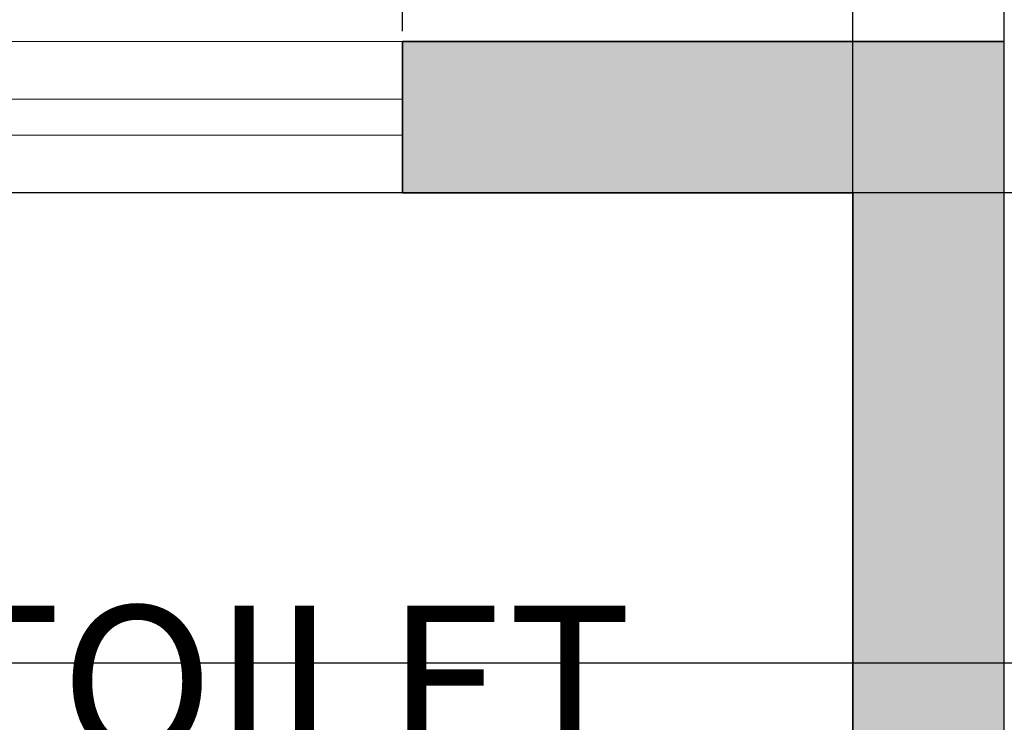
# Model space of a CAD drawing. Units: inches. Extents: x 2696 to 3240, y 1564 to 2310.
# Tile 62 of 76: x 2907 to 2966, y 2222 to 2264. Entities that reach past the tile are written whole.
import ezdxf

# ---------------------------------------------------------------- set-up
doc = ezdxf.new("R2010")
doc.units = ezdxf.units.IN
for name, color, linetype, lineweight in [('A-ANNO-DIMS', 3, 'Continuous', 18), ('A-AREA-IDEN', 7, 'Continuous', 18), ('A-WALL', 7, 'Continuous', 35), ('A-WALL-PATT', 9, 'Continuous', 13), ('WINDOW', 2, 'Continuous', 18)]:
    doc.layers.add(name, color=color, linetype=linetype, lineweight=lineweight)
doc.styles.add('TIMES NEW', font='times.ttf')
doc.styles.add('YQ_DIM', font='SUPEROS.SHX', dxfattribs={"width": 0.8, "bigfont": 'HZDX.SHX'})
doc.dimstyles.new('Siddhuu', dxfattribs={"dimtxt": 6, "dimasz": 2.5, "dimexe": 1.25, "dimexo": 0.625, "dimtad": 1, "dimdec": 1, "dimlunit": 4, "dimtxsty": 'TIMES NEW', "dimcen": 2.5, "dimclrd": 256, "dimclre": 1, "dimclrt": 7, "dimadec": 0, "dimazin": 0, "dimtfac": 1, "dimtdec": 1, "dimtmove": 0, "dimatfit": 3, "dimfxl": 1, "dimtolj": 1, "dimlwd": -1, "dimarcsym": 0})

# ---------------------------------------------------------------- blocks, each defined once
blk = doc.blocks.new('WD_WIN4')
for p, q in [((-0.5, 0.5), (0.5, 0.5)), ((-0.5, 0.12), (0.5, 0.12)), ((-0.5, -0.12), (0.5, -0.12)), ((-0.5, -0.5), (0.5, -0.5))]:
    blk.add_line(p, q)
blk = doc.blocks.new('*D9')
at = {"layer": 'A-ANNO-DIMS', "color": 0, "lineweight": -2, "transparency": 16777216}
for p, q in [((2745.611, 2262.826), (2745.611, 2282.188)), ((3199.611, 2262.826), (3199.611, 2282.188))]:
    blk.add_line(p, q, dxfattribs=at)
at = {"layer": 'A-ANNO-DIMS', "color": 0, "transparency": 16777216}
blk.add_line((2757.611, 2280.938), (3187.611, 2280.938), dxfattribs=at)
for points in [[(2757.611, 2282.938), (2757.611, 2278.938), (2745.611, 2280.938)], [(3187.611, 2282.938), (3187.611, 2278.938), (3199.611, 2280.938)]]:
    blk.add_solid(points, dxfattribs=at)
at = {"layer": 'Defpoints', "color": 0, "transparency": 16777216}
for p in [(3199.611, 2280.938), (2745.611, 2262.201), (3199.611, 2262.201)]:
    blk.add_point(p, dxfattribs=at)
at = {"layer": 'A-ANNO-DIMS', "color": 0, "transparency": 16777216, "insert": (2972.611, 2290.718), "char_height": 18, "attachment_point": 5, "style": 'TIMES NEW'}
blk.add_mtext("\\A1;36'", dxfattribs=at)
blk = doc.blocks.new('*D20')
at = {"layer": 'A-ANNO-DIMS', "color": 1, "lineweight": -2, "transparency": 16777216}
for p, q in [((2905.91, 2262.826), (2905.91, 2267.051)), ((2929.91, 2262.826), (2929.91, 2267.051))]:
    blk.add_line(p, q, dxfattribs=at)
at = {"layer": 'A-ANNO-DIMS', "transparency": 16777216}
for p, q in [((2905.91, 2265.801), (2844.76, 2265.801)), ((2927.41, 2265.801), (2908.41, 2265.801))]:
    blk.add_line(p, q, dxfattribs=at)
for points in [[(2908.41, 2266.218), (2908.41, 2265.384), (2905.91, 2265.801)], [(2927.41, 2266.218), (2927.41, 2265.384), (2929.91, 2265.801)]]:
    blk.add_solid(points, dxfattribs=at)
at = {"layer": 'Defpoints', "color": 0, "transparency": 16777216}
for p in [(2905.91, 2265.801), (2905.91, 2262.201), (2929.91, 2262.201)]:
    blk.add_point(p, dxfattribs=at)
at = {"layer": 'A-ANNO-DIMS', "color": 7, "transparency": 16777216, "insert": (2874.085, 2269.493), "char_height": 6, "attachment_point": 5, "style": 'TIMES NEW'}
blk.add_mtext('\\A1;WINDOW 2\'-0"', dxfattribs=at)
blk = doc.blocks.new('*D59')
at = {"layer": 'A-ANNO-DIMS', "color": 1, "lineweight": -2, "transparency": 16777216}
for p, q in [((2884.709, 1740.826), (2884.709, 2298.451)), ((2956.709, 1740.826), (2956.709, 2298.451))]:
    blk.add_line(p, q, dxfattribs=at)
at = {"layer": 'A-ANNO-DIMS', "transparency": 16777216}
blk.add_line((2887.209, 2297.201), (2954.209, 2297.201), dxfattribs=at)
for points in [[(2887.209, 2297.618), (2887.209, 2296.784), (2884.709, 2297.201)], [(2954.209, 2297.618), (2954.209, 2296.784), (2956.709, 2297.201)]]:
    blk.add_solid(points, dxfattribs=at)
at = {"layer": 'Defpoints', "color": 0, "transparency": 16777216}
for p in [(2956.709, 2297.201), (2884.709, 1740.201), (2956.709, 1740.201)]:
    blk.add_point(p, dxfattribs=at)
at = {"layer": 'A-ANNO-DIMS', "color": 7, "transparency": 16777216, "insert": (2920.709, 2300.878), "char_height": 6, "attachment_point": 5, "style": 'TIMES NEW'}
blk.add_mtext('\\A1;6\'-0"', dxfattribs=at)
blk = doc.blocks.new('*D61')
at = {"layer": 'A-ANNO-DIMS', "color": 1, "lineweight": -2, "transparency": 16777216}
for p, q in [((2965.709, 2141.326), (2965.709, 2298.451)), ((3044.302, 2141.326), (3044.302, 2298.451))]:
    blk.add_line(p, q, dxfattribs=at)
at = {"layer": 'A-ANNO-DIMS', "transparency": 16777216}
blk.add_line((2968.209, 2297.201), (3041.802, 2297.201), dxfattribs=at)
for points in [[(2968.209, 2297.618), (2968.209, 2296.784), (2965.709, 2297.201)], [(3041.802, 2297.618), (3041.802, 2296.784), (3044.302, 2297.201)]]:
    blk.add_solid(points, dxfattribs=at)
at = {"layer": 'Defpoints', "color": 0, "transparency": 16777216}
for p in [(3044.302, 2297.201), (2965.709, 2140.701), (3044.302, 2140.701)]:
    blk.add_point(p, dxfattribs=at)
at = {"layer": 'A-ANNO-DIMS', "color": 7, "transparency": 16777216, "insert": (3005.005, 2300.962), "char_height": 6, "attachment_point": 5, "style": 'TIMES NEW'}
blk.add_mtext('\\A1;6\'-6 1/2"', dxfattribs=at)
blk = doc.blocks.new('*D63')
at = {"layer": 'A-ANNO-DIMS', "color": 1, "lineweight": -2, "transparency": 16777216}
for p, q in [((2965.709, 1989.826), (2965.709, 2298.451)), ((3069.209, 1989.826), (3069.209, 2298.451))]:
    blk.add_line(p, q, dxfattribs=at)
at = {"layer": 'A-ANNO-DIMS', "transparency": 16777216}
blk.add_line((2968.209, 2297.201), (3066.709, 2297.201), dxfattribs=at)
for points in [[(2968.209, 2297.618), (2968.209, 2296.784), (2965.709, 2297.201)], [(3066.709, 2297.618), (3066.709, 2296.784), (3069.209, 2297.201)]]:
    blk.add_solid(points, dxfattribs=at)
at = {"layer": 'Defpoints', "color": 0, "transparency": 16777216}
for p in [(3069.209, 2297.201), (2965.709, 1989.201), (3069.209, 1989.201)]:
    blk.add_point(p, dxfattribs=at)
at = {"layer": 'A-ANNO-DIMS', "color": 7, "transparency": 16777216, "insert": (3017.459, 2300.962), "char_height": 6, "attachment_point": 5, "style": 'TIMES NEW'}
blk.add_mtext('\\A1;8\'-7 1/2"', dxfattribs=at)
blk = doc.blocks.new('*D70')
at = {"layer": 'A-ANNO-DIMS', "color": 1, "lineweight": -2, "transparency": 16777216}
for p, q in [((2929.91, 2262.826), (2929.91, 2298.451)), ((2965.709, 2262.826), (2965.709, 2298.451))]:
    blk.add_line(p, q, dxfattribs=at)
at = {"layer": 'A-ANNO-DIMS', "transparency": 16777216}
blk.add_line((2932.41, 2297.201), (2963.209, 2297.201), dxfattribs=at)
for points in [[(2932.41, 2297.618), (2932.41, 2296.784), (2929.91, 2297.201)], [(2963.209, 2297.618), (2963.209, 2296.784), (2965.709, 2297.201)]]:
    blk.add_solid(points, dxfattribs=at)
at = {"layer": 'Defpoints', "color": 0, "transparency": 16777216}
for p in [(2965.709, 2297.201), (2929.91, 2262.201), (2965.709, 2262.201)]:
    blk.add_point(p, dxfattribs=at)
at = {"layer": 'A-ANNO-DIMS', "color": 7, "transparency": 16777216, "insert": (2947.809, 2300.878), "char_height": 6, "attachment_point": 5, "style": 'TIMES NEW'}
blk.add_mtext('\\A1;3\'-0"', dxfattribs=at)
blk = doc.blocks.new('*D76')
at = {"layer": 'A-ANNO-DIMS', "color": 1, "lineweight": -2, "transparency": 16777216}
for p, q in [((3189.986, 2253.201), (2709.361, 2253.201)), ((3189.986, 2225.201), (2709.361, 2225.201))]:
    blk.add_line(p, q, dxfattribs=at)
at = {"layer": 'A-ANNO-DIMS', "transparency": 16777216}
blk.add_line((2710.611, 2250.701), (2710.611, 2227.701), dxfattribs=at)
for points in [[(2710.195, 2250.701), (2711.028, 2250.701), (2710.611, 2253.201)], [(2710.195, 2227.701), (2711.028, 2227.701), (2710.611, 2225.201)]]:
    blk.add_solid(points, dxfattribs=at)
at = {"layer": 'Defpoints', "color": 0, "transparency": 16777216}
for p in [(3190.611, 2253.201), (2710.611, 2225.201), (3190.611, 2225.201)]:
    blk.add_point(p, dxfattribs=at)
at = {"layer": 'A-ANNO-DIMS', "color": 7, "transparency": 16777216, "insert": (2706.986, 2239.201), "char_height": 6, "attachment_point": 5, "rotation": 90, "style": 'TIMES NEW'}
blk.add_mtext('\\A1;2\'-4"', dxfattribs=at)

msp = doc.modelspace()

# ---------------------------------------------------------------- hatches: boundary and pattern name
at = {"layer": 'A-WALL-PATT', "transparency": 33554556}
h = msp.add_hatch(color=256, dxfattribs=at)
h.dxf.hatch_style = 1
h.paths.add_polyline_path([(2879.111, 2253.201), (2905.91, 2253.201), (2905.91, 2262.201), (2841.889, 2262.201), (2841.889, 2253.201), (2870.111, 2253.201), (2870.111, 2176.601), (2965.709, 2176.601), (2965.709, 2206.701), (2973.583, 2206.701), (2973.583, 2215.701), (2965.709, 2215.701), (2965.709, 2262.201), (2929.91, 2262.201), (2929.91, 2253.201), (2956.709, 2253.201), (2956.709, 2185.601), (2879.111, 2185.601)])
h.paths.add_polyline_path([(2782.834, 2262.201), (2745.611, 2262.201), (2745.611, 2228.729), (2754.611, 2228.729), (2754.611, 2253.201), (2782.834, 2253.201)])
h.paths.add_polyline_path([(2754.611, 2136.201), (2965.709, 2136.201), (2965.709, 2145.201), (2879.111, 2145.201), (2879.111, 2147.074), (2877.34, 2147.074), (2870.111, 2147.074), (2870.111, 2145.201), (2754.611, 2145.201), (2754.611, 2169.674), (2745.611, 2169.674), (2745.611, 2000.201), (2754.611, 2000.201), (2754.611, 2019.201), (2849.083, 2019.201), (2849.083, 2023.701), (2841.209, 2023.701), (2841.209, 2051.827), (2836.709, 2051.827), (2836.709, 2023.701), (2754.611, 2023.701), (2754.611, 2091.201), (2836.709, 2091.201), (2836.709, 2087.827), (2841.209, 2087.827), (2841.209, 2095.701), (2754.611, 2095.701)])
h.paths.add_polyline_path([(2965.709, 2136.201), (2956.709, 2136.201), (2956.709, 2023.701), (2885.083, 2023.701), (2885.083, 2019.201), (2956.709, 2019.201), (2956.709, 1950.575), (2965.709, 1950.575), (2965.709, 1980.201), (2973.583, 1980.201), (2973.583, 1989.201), (2965.709, 1989.201)])
h.paths.add_polyline_path([(2754.611, 1906.701), (2880.209, 1906.701), (2884.709, 1906.701), (2956.709, 1906.701), (2956.709, 1792.701), (2944.709, 1792.701), (2944.709, 1783.701), (2956.709, 1783.701), (2956.709, 1740.201), (2884.709, 1740.201), (2884.709, 1783.701), (2896.709, 1783.701), (2896.709, 1792.701), (2884.709, 1792.701), (2884.709, 1846.701), (2880.209, 1846.701), (2880.209, 1740.201), (2754.611, 1740.201), (2754.611, 1777.201), (2745.611, 1777.201), (2745.611, 1692.701), (2754.611, 1692.701), (2754.611, 1731.201), (2956.709, 1731.201), (2956.709, 1723.327), (2965.709, 1723.327), (2965.709, 1884.201), (2973.583, 1884.201), (2973.583, 1893.201), (2965.709, 1893.201), (2965.709, 1914.575), (2956.709, 1914.575), (2956.709, 1911.201), (2754.611, 1911.201), (2754.611, 1930.201), (2745.611, 1930.201), (2745.611, 1817.201), (2754.611, 1817.201), (2754.611, 1854.201), (2826.611, 1854.201), (2826.611, 1868.827), (2822.111, 1868.827), (2822.111, 1858.701), (2754.611, 1858.701)])
h.paths.add_polyline_path([(2965.709, 1656.201), (3008.237, 1656.201), (3008.237, 1665.201), (2965.709, 1665.201), (2965.709, 1693.327), (2956.709, 1693.327), (2956.709, 1686.201), (2934.583, 1686.201), (2934.583, 1681.701), (2956.709, 1681.701), (2956.709, 1614.201), (2896.709, 1614.201), (2896.709, 1681.701), (2904.583, 1681.701), (2904.583, 1686.201), (2892.209, 1686.201), (2892.209, 1614.201), (2858.41, 1614.201), (2858.41, 1605.201), (2965.709, 1605.201)])
h.paths.add_polyline_path([(2788.41, 1614.201), (2754.611, 1614.201), (2754.611, 1652.701), (2745.611, 1652.701), (2745.611, 1605.201), (2788.41, 1605.201)])
h.paths.add_polyline_path([(3199.611, 1633.048), (3190.611, 1633.048), (3190.611, 1614.201), (3082.611, 1614.201), (3082.611, 1665.201), (3070.237, 1665.201), (3070.237, 1656.201), (3078.111, 1656.201), (3078.111, 1605.201), (3199.611, 1605.201)])
h.paths.add_polyline_path([(3199.611, 1702.048), (3190.611, 1702.048), (3190.611, 1699.701), (3106.611, 1699.701), (3106.611, 1747.701), (3190.611, 1747.701), (3190.611, 1752.201), (3082.611, 1752.201), (3082.611, 1760.075), (3078.111, 1760.075), (3078.111, 1747.701), (3102.111, 1747.701), (3102.111, 1699.701), (3078.111, 1699.701), (3078.111, 1695.201), (3190.611, 1695.201), (3190.611, 1676.355), (3199.611, 1676.355)])
h.paths.add_polyline_path([(3199.611, 1783.201), (3190.611, 1783.201), (3190.611, 1745.355), (3199.611, 1745.355)])
h.paths.add_polyline_path([(3082.611, 1884.201), (3190.611, 1884.201), (3190.611, 1853.201), (3199.611, 1853.201), (3199.611, 1901.701), (3190.611, 1901.701), (3190.611, 1893.201), (3005.583, 1893.201), (3005.583, 1891.281), (3005.583, 1884.201), (3078.111, 1884.201), (3078.111, 1792.075), (3082.611, 1792.075)])
h.paths.add_polyline_path([(3199.611, 1994.701), (3190.611, 1994.701), (3190.611, 1989.201), (3073.709, 1989.201), (3073.709, 2034.201), (3069.209, 2034.201), (3069.209, 1989.201), (3005.583, 1989.201), (3005.583, 1980.201), (3190.611, 1980.201), (3190.611, 1971.701), (3199.611, 1971.701)])
h.paths.add_polyline_path([(3199.611, 2155.201), (3190.611, 2155.201), (3190.611, 2064.701), (3199.611, 2064.701)])
h.paths.add_polyline_path([(3190.611, 2074.701), (3106.611, 2074.701), (3106.611, 2122.701), (3190.611, 2122.701), (3190.611, 2127.201), (3082.709, 2127.201), (3082.709, 2135.075), (3073.709, 2135.075), (3073.709, 2122.701), (3102.111, 2122.701), (3102.111, 2074.701), (3069.209, 2074.701), (3069.209, 2070.201), (3190.611, 2070.201)])
h.paths.add_polyline_path([(3082.709, 2253.201), (3190.611, 2253.201), (3190.611, 2225.201), (3199.611, 2225.201), (3199.611, 2262.201), (3073.709, 2262.201), (3073.709, 2215.701), (3035.583, 2215.701), (3035.583, 2206.701), (3073.709, 2206.701), (3073.709, 2171.075), (3082.709, 2171.075)])

# ---------------------------------------------------------------- linework, layer by layer
at = {"layer": 'A-WALL'}
for p, q in [((2929.91, 2262.201), (2929.91, 2253.201)), ((2929.91, 2262.201), (2965.709, 2262.201)), ((2929.91, 2253.201), (2929.91, 2262.201)), ((2929.91, 2253.201), (2956.709, 2253.201)), ((2956.709, 2185.601), (2956.709, 2253.201))]:
    msp.add_line(p, q, dxfattribs=at)

# ---------------------------------------------------------------- block references
at = {"layer": 'WINDOW', "xscale": 24, "yscale": 9, "zscale": 24, "rotation": 180}
msp.add_blockref('WD_WIN4', (2917.91, 2257.701), dxfattribs=at)

# ---------------------------------------------------------------- texts
at = {"layer": 'A-AREA-IDEN', "insert": (2902.228, 2228.623), "char_height": 9, "attachment_point": 1, "style": 'YQ_DIM'}
msp.add_mtext_dynamic_manual_height_columns('TOILET\\P5\'X5\'4.5"', width=48.00324, gutter_width=12.5, heights=[0], dxfattribs=at)

# ---------------------------------------------------------------- dimensions: what is measured, and where the dimension line sits
at = {"layer": 'A-ANNO-DIMS'}
for base, p1, p2, picture, middle in [((3044.302, 2297.201), (2965.709, 2140.701), (3044.302, 2140.701), '*D61', (3005.005, 2300.962)), ((3069.209, 2297.201), (2965.709, 1989.201), (3069.209, 1989.201), '*D63', (3017.459, 2300.962)), ((2956.709, 2297.201), (2884.709, 1740.201), (2956.709, 1740.201), '*D59', (2920.709, 2300.878)), ((2965.709, 2297.201), (2929.91, 2262.201), (2965.709, 2262.201), '*D70', (2947.809, 2300.878))]:
    dim = msp.add_linear_dim(base=base, p1=p1, p2=p2, dimstyle='Siddhuu', override={"dimdec": 1, "dimlfac": 1, "dimrnd": 0, "dimzin": 1, "dimdsep": 46, "dimlunit": 4, "dimfrac": 2}, dxfattribs=at)
    dim.commit()
    dim.dimension.update_dxf_attribs({"geometry": picture, "text_midpoint": middle})
dim = msp.add_linear_dim(base=(3199.611, 2280.938), p1=(2745.611, 2262.201), p2=(3199.611, 2262.201), text="36'", dimstyle='Siddhuu', override={"dimtxt": 18, "dimasz": 12, "dimclrd": 0, "dimclre": 0, "dimclrt": 0}, dxfattribs=at)
dim.commit()
dim.dimension.update_dxf_attribs({"geometry": '*D9', "text_midpoint": (2972.611, 2290.718)})
dim = msp.add_linear_dim(base=(2905.91, 2265.801), p1=(2929.91, 2262.201), p2=(2905.91, 2262.201), angle=180, text='WINDOW <>', dimstyle='Siddhuu', override={"dimdec": 1, "dimlfac": 1, "dimrnd": 0, "dimzin": 1, "dimdsep": 46, "dimlunit": 4, "dimfrac": 2}, dxfattribs=at)
dim.commit()
dim.dimension.update_dxf_attribs({"geometry": '*D20', "text_midpoint": (2874.085, 2269.493)})
dim = msp.add_linear_dim(base=(2710.611, 2225.201), p1=(3190.611, 2253.201), p2=(3190.611, 2225.201), angle=90, dimstyle='Siddhuu', override={"dimdec": 1, "dimlfac": 1, "dimrnd": 0, "dimzin": 1, "dimdsep": 46, "dimlunit": 4, "dimfrac": 2}, dxfattribs=at)
dim.commit()
dim.dimension.update_dxf_attribs({"geometry": '*D76', "text_midpoint": (2706.986, 2239.201)})

doc.saveas('drawing.dxf')
